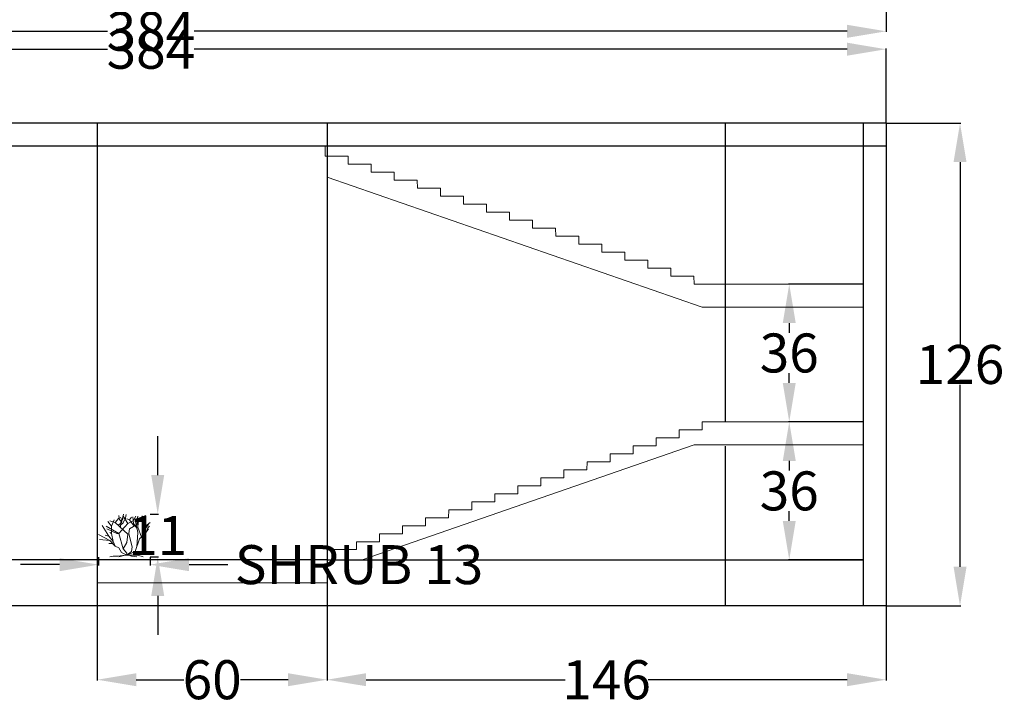
# Model space of a CAD drawing. Units: inches. Extents: x -107 to 647, y -210 to 500.
# Tile 3 of 7: x 183 to 440, y -210 to -31. Entities that reach past the tile are written whole.
import ezdxf

# ---------------------------------------------------------------- set-up
doc = ezdxf.new("R2010")
doc.units = ezdxf.units.IN
doc.header["$MEASUREMENT"] = 0
for name, color, linetype, lineweight in [('A-ANNO-DIMS', 2, 'Continuous', 18), ('A-ELEV', 30, 'Continuous', 25), ('A-ELEV-STRS', 7, 'Continuous', 18), ('L-PLNT', 3, 'Continuous', 13)]:
    doc.layers.add(name, color=color, linetype=linetype, lineweight=lineweight)
doc.styles.get("Standard").update_dxf_attribs({"font": 'arial.ttf'})
doc.dimstyles.get("Standard").update_dxf_attribs({"dimtxt": 10.18, "dimasz": 10.18, "dimexe": 0.18, "dimexo": 0.0625, "dimgap": 0.09, "dimtad": 0, "dimtih": 1, "dimtoh": 1, "dimdec": 0, "dimzin": 0, "dimdsep": 46, "dimlunit": 3, "dimtxsty": 'Standard', "dimcen": 0.09, "dimadec": 0, "dimazin": 0, "dimtfac": 1, "dimtdec": 0, "dimtofl": 0, "dimtmove": 0, "dimatfit": 3, "dimfxl": 1, "dimtolj": 1, "dimtzin": 0, "dimarcsym": 0})

# ---------------------------------------------------------------- blocks, each defined once
blk = doc.blocks.new('Shrub - elevation')
for p, q in [((-12.471, 19.775), (-12.898, 22.044)), ((-11.28, 19.619), (-12.104, 21.184)), ((-11.433, 18.289), (-10.457, 22.749)), ((-8.16, 17.76), (-10.56, 21.6)), ((-9.48, 19.775), (-8.992, 22.592)), ((-7.2, 19.68), (-6.24, 21.12)), ((-5.086, 17.741), (-5.513, 21.34)), ((-5.28, 19.2), (-3.84, 21.6)), ((-3.377, 18.602), (-2.888, 21.575)), ((-0.508, 21.888), (-0.081, 20.558)), ((-0.203, 19.149), (0.102, 21.34)), ((-0.02, 20.01), (0.896, 21.105)), ((0.041, 20.714), (1.384, 22.044)), ((0.102, 21.34), (0.835, 21.888)), ((-18.24, 11.04), (-21.755, 16.655)), ((-12.96, 12.48), (-19.68, 16.32)), ((-16.8, 16.32), (-18.72, 18.72)), ((-14.88, 18.24), (-17.76, 19.2)), ((-16.8, 16.32), (-15.36, 19.68)), ((-16.8, 12.48), (-16.8, 16.32)), ((-14.88, 18.24), (-12.96, 20.64)), ((-8.16, 12), (-14.88, 18.24)), ((-13.325, 16.724), (-11.433, 18.289)), ((-12.96, 12.48), (-8.16, 17.76)), ((-11.677, 19.071), (-12.471, 19.775)), ((-12.043, 15.628), (-11.921, 18.836)), ((-11.982, 16.802), (-10.579, 18.054)), ((-11.921, 18.836), (-10.64, 20.401)), ((-10.579, 18.054), (-9.846, 19.697)), ((-7.2, 19.68), (-8.64, 20.16)), ((-8.16, 17.76), (-5.28, 19.2)), ((-4.8, 16.32), (-7.2, 19.68)), ((-7.2, 14.88), (-3.84, 16.8)), ((-3.377, 15.315), (-5.086, 17.819)), ((-2.88, 12.96), (-4.32, 19.68)), ((-3.84, 16.8), (-0.96, 20.64)), ((-2.766, 16.802), (-3.377, 18.602)), ((-2.88, 15.84), (-2.4, 20.16)), ((-0.96, 10.56), (-2.88, 15.84)), ((0.346, 13.203), (-0.203, 19.149)), ((-0.142, 19.384), (0.59, 20.401)), ((0.346, 13.203), (1.323, 16.254)), ((1.323, 16.254), (3.642, 18.289)), ((1.44, 15.36), (2.88, 17.28)), ((2.4, 15.36), (3.36, 16.32)), ((-17.76, 8.64), (-23.663, 11.961)), ((-18.24, 11.04), (-20.16, 11.52)), ((-13.92, 12.48), (-19.2, 14.88)), ((-15.84, 8.16), (-18.24, 11.04)), ((-16.8, 12.48), (-17.76, 12.96)), ((-15.84, 8.16), (-16.8, 12.48)), ((-12.96, 12.48), (-13.92, 12.48)), ((-10.56, 4.32), (-12.96, 12.48)), ((-8.64, 7.68), (-8.16, 12)), ((-7.68, 12.48), (-7.2, 14.88)), ((-6.72, 8.64), (-7.68, 12.48)), ((-3.36, 5.28), (-2.88, 12.96)), ((-1.92, 9.6), (0.96, 12)), ((-0.48, 10.8), (0.346, 13.203)), ((0.96, 12), (1.44, 15.36)), ((0.96, 12), (2.88, 14.88)), ((1.92, 13.44), (2.4, 15.36)), ((-17.76, 8.64), (-23.128, 9.222)), ((-16.32, 7.2), (-18.24, 7.2)), ((-14.88, 5.76), (-17.76, 8.64)), ((-14.88, 5.76), (-15.84, 8.16)), ((-12.96, 4.8), (-14.88, 5.76)), ((-10.56, 4.32), (-8.64, 7.68)), ((-5.76, 5.28), (-6.72, 8.64)), ((-6.24, 2.88), (-5.76, 5.28)), ((-4.32, 2.88), (-1.92, 9.6)), ((-15.84, 0.48), (-17.76, 0)), ((-13.44, 0.48), (-15.84, 0.48)), ((-9.6, 0.96), (-13.44, 0.48)), ((-11.52, 2.4), (-12.96, 4.8)), ((-9.6, 0.96), (-12.96, 0)), ((-8.64, 0.96), (-11.52, 2.4)), ((-8.64, 1.92), (-10.56, 4.32)), ((-9.6, 0.96), (-7.68, 0.96)), ((-8.64, 0.96), (-4.32, 2.88)), ((-8.64, 0.96), (-6.24, 2.88)), ((-8.64, 0.96), (-8.64, 1.92)), ((-8.64, 0.96), (-2.88, 0.96)), ((-7.68, 0.96), (-6.24, 0.48)), ((-6.24, 0.48), (-3.36, 0)), ((-2.88, 0.96), (0, 0))]:
    blk.add_line(p, q)
blk = doc.blocks.new('*D70')
at = {"layer": 'A-ANNO-DIMS', "color": 0, "lineweight": -2, "transparency": 16777216}
for p, q in [((203.41, -171.38), (203.41, -173.51)), ((216.85, -171.38), (216.85, -173.51)), ((193.23, -173.33), (183.05, -173.33)), ((227.03, -173.33), (237.21, -173.33))]:
    blk.add_line(p, q, dxfattribs=at)
at = {"layer": 'A-ANNO-DIMS', "color": 0, "transparency": 16777216}
for points in [[(193.23, -171.64), (193.23, -175.03), (203.41, -173.33)], [(227.03, -171.64), (227.03, -175.03), (216.85, -173.33)]]:
    blk.add_solid(points, dxfattribs=at)
at = {"layer": 'Defpoints', "color": 0, "transparency": 16777216}
for p in [(203.41, -171.32), (216.85, -171.32), (216.85, -173.33)]:
    blk.add_point(p, dxfattribs=at)
at = {"layer": 'A-ANNO-DIMS', "color": 0, "transparency": 16777216, "insert": (271.43, -173.33), "char_height": 10.18, "attachment_point": 5}
blk.add_mtext('\\A1;SHRUB 13', dxfattribs=at)
blk = doc.blocks.new('*D71')
at = {"layer": 'A-ANNO-DIMS', "color": 0, "lineweight": -2, "transparency": 16777216}
for p, q in [((218.86, -149.94), (218.86, -139.76)), ((216.91, -160.12), (219.04, -160.12)), ((216.91, -171.32), (219.04, -171.32)), ((218.86, -181.5), (218.86, -191.68))]:
    blk.add_line(p, q, dxfattribs=at)
at = {"layer": 'A-ANNO-DIMS', "color": 0, "transparency": 16777216}
for points in [[(217.17, -149.94), (220.56, -149.94), (218.86, -160.12)], [(217.17, -181.5), (220.56, -181.5), (218.86, -171.32)]]:
    blk.add_solid(points, dxfattribs=at)
at = {"layer": 'Defpoints', "color": 0, "transparency": 16777216}
for p in [(216.85, -160.12), (218.86, -160.12), (216.85, -171.32)]:
    blk.add_point(p, dxfattribs=at)
at = {"layer": 'A-ANNO-DIMS', "color": 0, "transparency": 16777216, "insert": (218.86, -165.72), "char_height": 10.18, "attachment_point": 5}
blk.add_mtext('\\A1;11', dxfattribs=at)
blk = doc.blocks.new('*D72')
at = {"layer": 'A-ANNO-DIMS', "color": 0, "lineweight": -2, "transparency": 16777216}
for p, q in [((25.08, 2.26), (25.08, -34.27)), ((409.08, 2.26), (409.08, -34.27)), ((35.26, -34.09), (205.77, -34.09)), ((398.9, -34.09), (228.39, -34.09))]:
    blk.add_line(p, q, dxfattribs=at)
at = {"layer": 'A-ANNO-DIMS', "color": 0, "transparency": 16777216}
for points in [[(35.26, -32.39), (35.26, -35.79), (25.08, -34.09)], [(398.9, -32.39), (398.9, -35.79), (409.08, -34.09)]]:
    blk.add_solid(points, dxfattribs=at)
at = {"layer": 'Defpoints', "color": 0, "transparency": 16777216}
for p in [(25.08, 2.33), (409.08, 2.33), (409.08, -34.09)]:
    blk.add_point(p, dxfattribs=at)
at = {"layer": 'A-ANNO-DIMS', "color": 0, "transparency": 16777216, "insert": (217.08, -34.09), "char_height": 10.18, "attachment_point": 5}
blk.add_mtext('\\A1;384', dxfattribs=at)
blk = doc.blocks.new('*D84')
at = {"layer": 'A-ANNO-DIMS', "color": 0, "lineweight": -2, "transparency": 16777216}
for p, q in [((25.08, -58.01), (25.08, -38.59)), ((35.26, -38.77), (205.77, -38.77)), ((398.9, -38.77), (228.39, -38.77)), ((409.08, -58.01), (409.08, -38.59))]:
    blk.add_line(p, q, dxfattribs=at)
at = {"layer": 'A-ANNO-DIMS', "color": 0, "transparency": 16777216}
for points in [[(35.26, -37.07), (35.26, -40.46), (25.08, -38.77)], [(398.9, -37.07), (398.9, -40.46), (409.08, -38.77)]]:
    blk.add_solid(points, dxfattribs=at)
at = {"layer": 'Defpoints', "color": 0, "transparency": 16777216}
for p in [(409.08, -38.77), (25.08, -58.07), (409.08, -58.07)]:
    blk.add_point(p, dxfattribs=at)
at = {"layer": 'A-ANNO-DIMS', "color": 0, "transparency": 16777216, "insert": (217.08, -38.77), "char_height": 10.18, "attachment_point": 5}
blk.add_mtext('\\A1;384', dxfattribs=at)
blk = doc.blocks.new('*D85')
at = {"layer": 'A-ANNO-DIMS', "color": 0, "lineweight": -2, "transparency": 16777216}
for p, q in [((409.14, -58.07), (428.56, -58.07)), ((428.38, -68.25), (428.38, -115.78)), ((428.38, -173.89), (428.38, -126.36)), ((409.14, -184.07), (428.56, -184.07))]:
    blk.add_line(p, q, dxfattribs=at)
at = {"layer": 'A-ANNO-DIMS', "color": 0, "transparency": 16777216}
for points in [[(426.69, -68.25), (430.08, -68.25), (428.38, -58.07)], [(426.69, -173.89), (430.08, -173.89), (428.38, -184.07)]]:
    blk.add_solid(points, dxfattribs=at)
at = {"layer": 'Defpoints', "color": 0, "transparency": 16777216}
for p in [(409.08, -58.07), (428.38, -58.07), (409.08, -184.07)]:
    blk.add_point(p, dxfattribs=at)
at = {"layer": 'A-ANNO-DIMS', "color": 0, "transparency": 16777216, "insert": (428.38, -121.07), "char_height": 10.18, "attachment_point": 5}
blk.add_mtext('\\A1;126', dxfattribs=at)
blk = doc.blocks.new('*D92')
at = {"layer": 'A-ANNO-DIMS', "color": 0, "lineweight": -2, "transparency": 16777216}
for p, q in [((203.08, -184.13), (203.08, -203.55)), ((263.08, -184.13), (263.08, -203.55)), ((213.26, -203.37), (225.69, -203.37)), ((252.9, -203.37), (240.47, -203.37))]:
    blk.add_line(p, q, dxfattribs=at)
at = {"layer": 'A-ANNO-DIMS', "color": 0, "transparency": 16777216}
for points in [[(213.26, -201.67), (213.26, -205.06), (203.08, -203.37)], [(252.9, -201.67), (252.9, -205.06), (263.08, -203.37)]]:
    blk.add_solid(points, dxfattribs=at)
at = {"layer": 'Defpoints', "color": 0, "transparency": 16777216}
for p in [(203.08, -184.07), (263.08, -184.07), (263.08, -203.37)]:
    blk.add_point(p, dxfattribs=at)
at = {"layer": 'A-ANNO-DIMS', "color": 0, "transparency": 16777216, "insert": (233.08, -203.37), "char_height": 10.18, "attachment_point": 5}
blk.add_mtext('\\A1;60', dxfattribs=at)
blk = doc.blocks.new('*D93')
at = {"layer": 'A-ANNO-DIMS', "color": 0, "lineweight": -2, "transparency": 16777216}
for p, q in [((263.08, -184.13), (263.08, -203.55)), ((409.08, -184.13), (409.08, -203.55)), ((273.26, -203.37), (325.23, -203.37)), ((398.9, -203.37), (346.94, -203.37))]:
    blk.add_line(p, q, dxfattribs=at)
at = {"layer": 'A-ANNO-DIMS', "color": 0, "transparency": 16777216}
for points in [[(273.26, -201.67), (273.26, -205.06), (263.08, -203.37)], [(398.9, -201.67), (398.9, -205.06), (409.08, -203.37)]]:
    blk.add_solid(points, dxfattribs=at)
at = {"layer": 'Defpoints', "color": 0, "transparency": 16777216}
for p in [(263.08, -184.07), (409.08, -184.07), (409.08, -203.37)]:
    blk.add_point(p, dxfattribs=at)
at = {"layer": 'A-ANNO-DIMS', "color": 0, "transparency": 16777216, "insert": (336.08, -203.37), "char_height": 10.18, "attachment_point": 5}
blk.add_mtext('\\A1;146', dxfattribs=at)
blk = doc.blocks.new('*D95')
at = {"layer": 'A-ANNO-DIMS', "color": 0, "lineweight": -2, "transparency": 16777216}
for p, q in [((5.78, -161.89), (5.78, -151.71)), ((263.02, -172.07), (5.6, -172.07)), ((263.02, -184.07), (5.6, -184.07)), ((5.78, -194.25), (5.78, -204.43))]:
    blk.add_line(p, q, dxfattribs=at)
at = {"layer": 'A-ANNO-DIMS', "color": 0, "transparency": 16777216}
for points in [[(4.09, -161.89), (7.48, -161.89), (5.78, -172.07)], [(4.09, -194.25), (7.48, -194.25), (5.78, -184.07)]]:
    blk.add_solid(points, dxfattribs=at)
at = {"layer": 'Defpoints', "color": 0, "transparency": 16777216}
for p in [(5.78, -172.07), (263.08, -172.07), (263.08, -184.07)]:
    blk.add_point(p, dxfattribs=at)
at = {"layer": 'A-ANNO-DIMS', "color": 0, "transparency": 16777216, "insert": (5.78, -178.07), "char_height": 10.18, "attachment_point": 5}
blk.add_mtext('\\A1;12', dxfattribs=at)
blk = doc.blocks.new('*D96')
at = {"layer": 'A-ANNO-DIMS', "color": 0, "lineweight": -2, "transparency": 16777216}
for p, q in [((403.02, -136.07), (383.6, -136.07)), ((383.78, -146.25), (383.78, -148.78)), ((383.78, -161.89), (383.78, -159.36)), ((403.02, -172.07), (383.6, -172.07))]:
    blk.add_line(p, q, dxfattribs=at)
at = {"layer": 'A-ANNO-DIMS', "color": 0, "transparency": 16777216}
for points in [[(382.09, -146.25), (385.48, -146.25), (383.78, -136.07)], [(382.09, -161.89), (385.48, -161.89), (383.78, -172.07)]]:
    blk.add_solid(points, dxfattribs=at)
at = {"layer": 'Defpoints', "color": 0, "transparency": 16777216}
for p in [(383.78, -136.07), (403.08, -136.07), (403.08, -172.07)]:
    blk.add_point(p, dxfattribs=at)
at = {"layer": 'A-ANNO-DIMS', "color": 0, "transparency": 16777216, "insert": (383.78, -154.07), "char_height": 10.18, "attachment_point": 5}
blk.add_mtext('\\A1;36', dxfattribs=at)
blk = doc.blocks.new('*D97')
at = {"layer": 'A-ANNO-DIMS', "color": 0, "lineweight": -2, "transparency": 16777216}
for p, q in [((403.02, -100.07), (383.6, -100.07)), ((383.78, -110.25), (383.78, -112.78)), ((383.78, -125.89), (383.78, -123.36)), ((403.02, -136.07), (383.6, -136.07))]:
    blk.add_line(p, q, dxfattribs=at)
at = {"layer": 'A-ANNO-DIMS', "color": 0, "transparency": 16777216}
for points in [[(382.09, -110.25), (385.48, -110.25), (383.78, -100.07)], [(382.09, -125.89), (385.48, -125.89), (383.78, -136.07)]]:
    blk.add_solid(points, dxfattribs=at)
at = {"layer": 'Defpoints', "color": 0, "transparency": 16777216}
for p in [(383.78, -100.07), (403.08, -100.07), (403.08, -136.07)]:
    blk.add_point(p, dxfattribs=at)
at = {"layer": 'A-ANNO-DIMS', "color": 0, "transparency": 16777216, "insert": (383.78, -118.07), "char_height": 10.18, "attachment_point": 5}
blk.add_mtext('\\A1;36', dxfattribs=at)

msp = doc.modelspace()

# ---------------------------------------------------------------- linework, layer by layer
at = {"layer": 'A-ELEV'}
for p, q in [((409.082, -58.068), (25.082, -58.068)), ((203.082, -58.068), (203.082, -184.068)), ((263.082, -58.068), (263.082, -184.068)), ((367.082, -58.068), (367.082, -136.068)), ((403.082, -58.068), (403.082, -184.068)), ((409.082, -58.068), (409.082, -184.068)), ((409.082, -64.068), (25.082, -64.068)), ((301.082, -64.068), (295.082, -64.068)), ((367.082, -142.417), (367.082, -184.068)), ((263.082, -172.068), (403.082, -172.068)), ((409.082, -184.068), (25.082, -184.068))]:
    msp.add_line(p, q, dxfattribs=at)
at = {"layer": 'A-ELEV-STRS'}
for p, q in [((263.082, -72.145), (361.082, -106.068)), ((403.082, -100.068), (358.92, -100.068)), ((403.082, -100.068), (367.082, -100.068)), ((361.082, -106.068), (367.082, -106.068)), ((403.082, -106.068), (366.073, -106.068)), ((403.082, -106.068), (367.082, -106.068)), ((361.082, -136.068), (361.061, -138.152)), ((367.082, -136.068), (361.082, -136.068)), ((367.082, -136.068), (403.082, -136.068)), ((355.061, -138.152), (355.04, -140.236)), ((361.061, -138.152), (355.061, -138.152)), ((349.04, -140.236), (349.019, -142.32)), ((355.04, -140.236), (349.04, -140.236)), ((358.92, -142.068), (272.253, -172.068)), ((343.019, -142.32), (342.998, -144.404)), ((349.019, -142.32), (343.019, -142.32)), ((358.92, -142.068), (403.082, -142.068)), ((330.977, -146.489), (330.956, -148.573)), ((336.977, -146.489), (330.977, -146.489)), ((336.998, -144.404), (336.977, -146.489)), ((342.998, -144.404), (336.998, -144.404)), ((324.956, -148.573), (324.935, -150.657)), ((330.956, -148.573), (324.956, -148.573)), ((318.935, -150.657), (318.914, -152.741)), ((324.935, -150.657), (318.935, -150.657)), ((312.914, -152.741), (312.894, -154.825)), ((318.914, -152.741), (312.914, -152.741)), ((306.894, -154.825), (306.873, -156.909)), ((312.894, -154.825), (306.894, -154.825)), ((294.852, -158.994), (294.831, -161.078)), ((300.852, -158.994), (294.852, -158.994)), ((300.873, -156.909), (300.852, -158.994)), ((306.873, -156.909), (300.873, -156.909)), ((288.831, -161.078), (288.81, -163.162)), ((294.831, -161.078), (288.831, -161.078)), ((282.81, -163.162), (282.789, -165.246)), ((288.81, -163.162), (282.81, -163.162)), ((276.789, -165.246), (276.768, -167.33)), ((282.789, -165.246), (276.789, -165.246)), ((264.747, -169.414), (264.72, -172.068)), ((270.747, -169.414), (264.747, -169.414)), ((270.768, -167.33), (270.747, -169.414)), ((276.768, -167.33), (270.768, -167.33)), ((263.082, -172.068), (203.082, -172.068)), ((263.082, -178.068), (203.082, -178.068))]:
    msp.add_line(p, q, dxfattribs=at)
msp.add_lwpolyline([(262.558, -64.068), (262.585, -66.721), (268.585, -66.721), (268.606, -68.805), (274.606, -68.805), (274.627, -70.889), (280.627, -70.889), (280.648, -72.974), (286.648, -72.974), (286.669, -75.058), (292.669, -75.058), (292.69, -77.142), (298.69, -77.142), (298.71, -79.226), (304.71, -79.226), (304.731, -81.31), (310.731, -81.31), (310.752, -83.394), (316.752, -83.394), (316.773, -85.479), (322.773, -85.479), (322.794, -87.563), (328.794, -87.563), (328.815, -89.647), (334.815, -89.647), (334.836, -91.731), (340.836, -91.731), (340.857, -93.815), (346.857, -93.815), (346.878, -95.899), (352.878, -95.899), (352.899, -97.984), (358.899, -97.984), (358.92, -100.068)], dxfattribs=at)

# ---------------------------------------------------------------- block references
at = {"layer": 'L-PLNT', "xscale": 0.4922175425746209, "yscale": 0.4922175425746209, "zscale": 0.4922175425746209}
msp.add_blockref('Shrub - elevation', (215.054, -171.319), dxfattribs=at)

# ---------------------------------------------------------------- dimensions: what is measured, and where the dimension line sits
at = {"layer": 'A-ANNO-DIMS'}
for base, p1, p2, picture, middle in [((409.082, -34.091), (25.082, 2.325), (409.082, 2.325), '*D72', (217.082, -34.091)), ((409.082, -38.768), (25.082, -58.068), (409.082, -58.068), '*D84', (217.082, -38.768)), ((263.082, -203.368), (203.082, -184.068), (263.082, -184.068), '*D92', (233.082, -203.368)), ((409.082, -203.368), (263.082, -184.068), (409.082, -184.068), '*D93', (336.082, -203.368))]:
    dim = msp.add_linear_dim(base=base, p1=p1, p2=p2, dimstyle='Standard', override={"dimdec": 0, "dimlfac": 1, "dimrnd": 0, "dimzin": 0, "dimdsep": 46, "dimlunit": 2}, dxfattribs=at)
    dim.commit()
    dim.dimension.update_dxf_attribs({"geometry": picture, "text_midpoint": middle})
for base, p1, p2, picture, middle in [((428.382, -58.068), (409.082, -184.068), (409.082, -58.068), '*D85', (428.382, -121.068)), ((383.782, -100.068), (403.082, -136.068), (403.082, -100.068), '*D97', (383.782, -118.068)), ((383.782, -136.068), (403.082, -172.068), (403.082, -136.068), '*D96', (383.782, -154.068)), ((218.862, -160.121), (216.846, -171.319), (216.846, -160.121), '*D71', (218.862, -165.72)), ((5.782, -172.068), (263.082, -184.068), (263.082, -172.068), '*D95', (5.782, -178.068))]:
    dim = msp.add_linear_dim(base=base, p1=p1, p2=p2, angle=90, dimstyle='Standard', override={"dimdec": 0, "dimlfac": 1, "dimrnd": 0, "dimzin": 0, "dimdsep": 46, "dimlunit": 2}, dxfattribs=at)
    dim.commit()
    dim.dimension.update_dxf_attribs({"geometry": picture, "text_midpoint": middle})
dim = msp.add_linear_dim(base=(216.846, -173.335), p1=(203.406, -171.319), p2=(216.846, -171.319), text='SHRUB <>', dimstyle='Standard', override={"dimdec": 0, "dimlfac": 1, "dimrnd": 0, "dimzin": 0, "dimdsep": 46, "dimlunit": 2}, dxfattribs=at)
dim.commit()
dim.dimension.update_dxf_attribs({"geometry": '*D70', "text_midpoint": (271.43, -173.335)})

doc.saveas('drawing.dxf')
